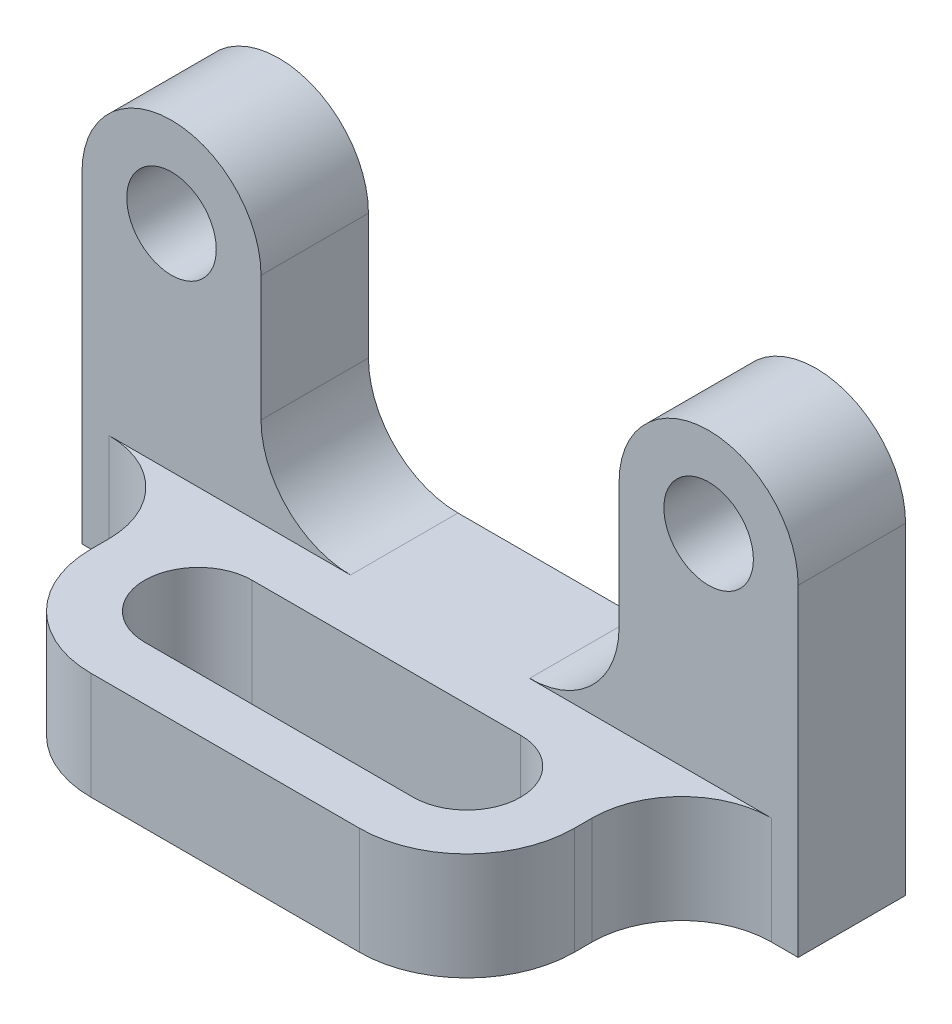
ISO-10303-21;
HEADER;
FILE_DESCRIPTION(('STEP AP214'),'2;1');
FILE_NAME('part.step','',(''),(''),'','','');
FILE_SCHEMA(('AUTOMOTIVE_DESIGN { 1 0 10303 214 1 1 1 1 }'));
ENDSEC;
DATA;
#1=APPLICATION_CONTEXT('core data for automotive mechanical design processes');
#2=APPLICATION_PROTOCOL_DEFINITION('international standard','automotive_design',2000,#1);
#3=PRODUCT_CONTEXT('',#1,'mechanical');
#4=PRODUCT('Part','Part','',(#3));
#5=PRODUCT_RELATED_PRODUCT_CATEGORY('part','',(#4));
#6=PRODUCT_DEFINITION_FORMATION('','',#4);
#7=PRODUCT_DEFINITION_CONTEXT('part definition',#1,'design');
#8=PRODUCT_DEFINITION('design','',#6,#7);
#9=PRODUCT_DEFINITION_SHAPE('','',#8);
#10=(LENGTH_UNIT() NAMED_UNIT(*) SI_UNIT(.MILLI.,.METRE.));
#11=(NAMED_UNIT(*) PLANE_ANGLE_UNIT() SI_UNIT($,.RADIAN.));
#12=(NAMED_UNIT(*) SI_UNIT($,.STERADIAN.) SOLID_ANGLE_UNIT());
#13=UNCERTAINTY_MEASURE_WITH_UNIT(LENGTH_MEASURE(1.E-05),#10,'distance_accuracy_value','');
#14=(GEOMETRIC_REPRESENTATION_CONTEXT(3) GLOBAL_UNCERTAINTY_ASSIGNED_CONTEXT((#13)) GLOBAL_UNIT_ASSIGNED_CONTEXT((#10,
#11,#12)) REPRESENTATION_CONTEXT('',''));
#15=CARTESIAN_POINT('',(0.,0.,0.));
#16=DIRECTION('',(0.,0.,1.));
#17=DIRECTION('',(1.,0.,0.));
#18=AXIS2_PLACEMENT_3D('',#15,#16,#17);
#19=CARTESIAN_POINT('',(0.,0.,6.));
#20=DIRECTION('',(0.,0.,1.));
#21=DIRECTION('',(1.,0.,0.));
#22=AXIS2_PLACEMENT_3D('',#19,#20,#21);
#23=PLANE('',#22);
#24=CARTESIAN_POINT('',(-15.,18.,6.));
#25=DIRECTION('',(0.,0.,1.));
#26=DIRECTION('',(1.,0.,0.));
#27=AXIS2_PLACEMENT_3D('',#24,#25,#26);
#28=CIRCLE('',#27,2.5);
#29=CARTESIAN_POINT('',(-12.5,18.,6.));
#30=VERTEX_POINT('',#29);
#31=EDGE_CURVE('E474',#30,#30,#28,.T.);
#32=ORIENTED_EDGE('',*,*,#31,.F.);
#33=EDGE_LOOP('',(#32));
#34=FACE_BOUND('',#33,.T.);
#35=DIRECTION('',(1.,0.,0.));
#36=VECTOR('',#35,1.);
#37=CARTESIAN_POINT('',(0.,0.,6.));
#38=LINE('',#37,#36);
#39=CARTESIAN_POINT('',(-20.,0.,6.));
#40=VERTEX_POINT('',#39);
#41=CARTESIAN_POINT('',(-18.5,0.,6.));
#42=VERTEX_POINT('',#41);
#43=EDGE_CURVE('E273',#40,#42,#38,.T.);
#44=ORIENTED_EDGE('',*,*,#43,.T.);
#45=DIRECTION('',(0.,-1.,0.));
#46=VECTOR('',#45,1.);
#47=CARTESIAN_POINT('',(-18.5,0.,6.));
#48=LINE('',#47,#46);
#49=CARTESIAN_POINT('',(-18.5,6.,6.));
#50=VERTEX_POINT('',#49);
#51=EDGE_CURVE('E359',#42,#50,#48,.F.);
#52=ORIENTED_EDGE('',*,*,#51,.T.);
#53=DIRECTION('',(-1.,0.,0.));
#54=VECTOR('',#53,1.);
#55=CARTESIAN_POINT('',(-13.5,6.,6.));
#56=LINE('',#55,#54);
#57=CARTESIAN_POINT('',(-5.,6.,6.));
#58=VERTEX_POINT('',#57);
#59=EDGE_CURVE('E243',#58,#50,#56,.T.);
#60=ORIENTED_EDGE('',*,*,#59,.F.);
#61=CARTESIAN_POINT('',(-5.,11.,6.));
#62=DIRECTION('',(0.,0.,1.));
#63=DIRECTION('',(1.,0.,0.));
#64=AXIS2_PLACEMENT_3D('',#61,#62,#63);
#65=CIRCLE('',#64,5.);
#66=CARTESIAN_POINT('',(-10.,11.,6.));
#67=VERTEX_POINT('',#66);
#68=EDGE_CURVE('E328',#58,#67,#65,.F.);
#69=ORIENTED_EDGE('',*,*,#68,.T.);
#70=DIRECTION('',(0.,-1.,0.));
#71=VECTOR('',#70,1.);
#72=CARTESIAN_POINT('',(-10.,0.,6.));
#73=LINE('',#72,#71);
#74=CARTESIAN_POINT('',(-10.,18.,6.));
#75=VERTEX_POINT('',#74);
#76=EDGE_CURVE('E264',#75,#67,#73,.T.);
#77=ORIENTED_EDGE('',*,*,#76,.F.);
#78=CARTESIAN_POINT('',(-15.,18.,6.));
#79=DIRECTION('',(0.,0.,1.));
#80=DIRECTION('',(1.,0.,0.));
#81=AXIS2_PLACEMENT_3D('',#78,#79,#80);
#82=CIRCLE('',#81,5.);
#83=CARTESIAN_POINT('',(-20.,18.,6.));
#84=VERTEX_POINT('',#83);
#85=EDGE_CURVE('E268',#75,#84,#82,.T.);
#86=ORIENTED_EDGE('',*,*,#85,.T.);
#87=DIRECTION('',(0.,1.,0.));
#88=VECTOR('',#87,1.);
#89=CARTESIAN_POINT('',(-20.,0.,6.));
#90=LINE('',#89,#88);
#91=EDGE_CURVE('E269',#40,#84,#90,.T.);
#92=ORIENTED_EDGE('',*,*,#91,.F.);
#93=EDGE_LOOP('',(#44,#52,#60,#69,#77,#86,#92));
#94=FACE_BOUND('',#93,.T.);
#95=ADVANCED_FACE('F44',(#34,#94),#23,.T.);
#96=CARTESIAN_POINT('',(20.,0.,6.));
#97=DIRECTION('',(-1.,0.,0.));
#98=DIRECTION('',(0.,0.,1.));
#99=AXIS2_PLACEMENT_3D('',#96,#97,#98);
#100=PLANE('',#99);
#101=DIRECTION('',(0.,1.,0.));
#102=VECTOR('',#101,1.);
#103=CARTESIAN_POINT('',(20.,0.,0.));
#104=LINE('',#103,#102);
#105=CARTESIAN_POINT('',(20.,0.,0.));
#106=VERTEX_POINT('',#105);
#107=CARTESIAN_POINT('',(20.,18.,0.));
#108=VERTEX_POINT('',#107);
#109=EDGE_CURVE('E254',#106,#108,#104,.T.);
#110=ORIENTED_EDGE('',*,*,#109,.T.);
#111=DIRECTION('',(0.,0.,-1.));
#112=VECTOR('',#111,1.);
#113=CARTESIAN_POINT('',(20.,18.,6.));
#114=LINE('',#113,#112);
#115=CARTESIAN_POINT('',(20.,18.,6.));
#116=VERTEX_POINT('',#115);
#117=EDGE_CURVE('E310',#116,#108,#114,.T.);
#118=ORIENTED_EDGE('',*,*,#117,.F.);
#119=DIRECTION('',(0.,1.,0.));
#120=VECTOR('',#119,1.);
#121=CARTESIAN_POINT('',(20.,0.,6.));
#122=LINE('',#121,#120);
#123=CARTESIAN_POINT('',(20.,0.,6.));
#124=VERTEX_POINT('',#123);
#125=EDGE_CURVE('E258',#124,#116,#122,.T.);
#126=ORIENTED_EDGE('',*,*,#125,.F.);
#127=DIRECTION('',(0.,0.,-1.));
#128=VECTOR('',#127,1.);
#129=CARTESIAN_POINT('',(20.,0.,6.));
#130=LINE('',#129,#128);
#131=EDGE_CURVE('E280',#124,#106,#130,.T.);
#132=ORIENTED_EDGE('',*,*,#131,.T.);
#133=EDGE_LOOP('',(#110,#118,#126,#132));
#134=FACE_BOUND('',#133,.T.);
#135=ADVANCED_FACE('F421',(#134),#100,.F.);
#136=CARTESIAN_POINT('',(15.,18.,6.));
#137=DIRECTION('',(0.,0.,-1.));
#138=DIRECTION('',(-1.,0.,0.));
#139=AXIS2_PLACEMENT_3D('',#136,#137,#138);
#140=CYLINDRICAL_SURFACE('',#139,5.);
#141=CARTESIAN_POINT('',(15.,18.,0.));
#142=DIRECTION('',(0.,0.,1.));
#143=DIRECTION('',(1.,0.,0.));
#144=AXIS2_PLACEMENT_3D('',#141,#142,#143);
#145=CIRCLE('',#144,5.);
#146=CARTESIAN_POINT('',(10.,18.,0.));
#147=VERTEX_POINT('',#146);
#148=EDGE_CURVE('E278',#108,#147,#145,.T.);
#149=ORIENTED_EDGE('',*,*,#148,.T.);
#150=DIRECTION('',(0.,0.,-1.));
#151=VECTOR('',#150,1.);
#152=CARTESIAN_POINT('',(10.,18.,6.));
#153=LINE('',#152,#151);
#154=CARTESIAN_POINT('',(10.,18.,6.));
#155=VERTEX_POINT('',#154);
#156=EDGE_CURVE('E308',#155,#147,#153,.T.);
#157=ORIENTED_EDGE('',*,*,#156,.F.);
#158=CARTESIAN_POINT('',(15.,18.,6.));
#159=DIRECTION('',(0.,0.,1.));
#160=DIRECTION('',(1.,0.,0.));
#161=AXIS2_PLACEMENT_3D('',#158,#159,#160);
#162=CIRCLE('',#161,5.);
#163=EDGE_CURVE('E259',#116,#155,#162,.T.);
#164=ORIENTED_EDGE('',*,*,#163,.F.);
#165=ORIENTED_EDGE('',*,*,#117,.T.);
#166=EDGE_LOOP('',(#149,#157,#164,#165));
#167=FACE_BOUND('',#166,.T.);
#168=ADVANCED_FACE('F416',(#167),#140,.T.);
#169=CARTESIAN_POINT('',(10.,0.,6.));
#170=DIRECTION('',(-1.,0.,0.));
#171=DIRECTION('',(0.,0.,1.));
#172=AXIS2_PLACEMENT_3D('',#169,#170,#171);
#173=PLANE('',#172);
#174=DIRECTION('',(0.,1.,0.));
#175=VECTOR('',#174,1.);
#176=CARTESIAN_POINT('',(10.,0.,0.));
#177=LINE('',#176,#175);
#178=CARTESIAN_POINT('',(10.,11.,0.));
#179=VERTEX_POINT('',#178);
#180=EDGE_CURVE('E283',#179,#147,#177,.T.);
#181=ORIENTED_EDGE('',*,*,#180,.F.);
#182=DIRECTION('',(0.,0.,-1.));
#183=VECTOR('',#182,1.);
#184=CARTESIAN_POINT('',(10.,11.,6.));
#185=LINE('',#184,#183);
#186=CARTESIAN_POINT('',(10.,11.,6.));
#187=VERTEX_POINT('',#186);
#188=EDGE_CURVE('E318',#179,#187,#185,.F.);
#189=ORIENTED_EDGE('',*,*,#188,.T.);
#190=DIRECTION('',(0.,1.,0.));
#191=VECTOR('',#190,1.);
#192=CARTESIAN_POINT('',(10.,0.,6.));
#193=LINE('',#192,#191);
#194=EDGE_CURVE('E263',#187,#155,#193,.T.);
#195=ORIENTED_EDGE('',*,*,#194,.T.);
#196=ORIENTED_EDGE('',*,*,#156,.T.);
#197=EDGE_LOOP('',(#181,#189,#195,#196));
#198=FACE_BOUND('',#197,.T.);
#199=ADVANCED_FACE('F411',(#198),#173,.T.);
#200=CARTESIAN_POINT('',(0.,6.,6.));
#201=DIRECTION('',(0.,1.,0.));
#202=DIRECTION('',(0.,0.,1.));
#203=AXIS2_PLACEMENT_3D('',#200,#201,#202);
#204=PLANE('',#203);
#205=CARTESIAN_POINT('',(-7.5,6.,12.));
#206=DIRECTION('',(0.,1.,0.));
#207=DIRECTION('',(0.,0.,1.));
#208=AXIS2_PLACEMENT_3D('',#205,#206,#207);
#209=CIRCLE('',#208,3.);
#210=CARTESIAN_POINT('',(-7.5,6.,9.));
#211=VERTEX_POINT('',#210);
#212=CARTESIAN_POINT('',(-7.5,6.,15.));
#213=VERTEX_POINT('',#212);
#214=EDGE_CURVE('E58',#211,#213,#209,.T.);
#215=ORIENTED_EDGE('',*,*,#214,.F.);
#216=DIRECTION('',(-1.,0.,0.));
#217=VECTOR('',#216,1.);
#218=CARTESIAN_POINT('',(-7.5,6.,9.));
#219=LINE('',#218,#217);
#220=CARTESIAN_POINT('',(7.5,6.,9.));
#221=VERTEX_POINT('',#220);
#222=EDGE_CURVE('E211',#221,#211,#219,.T.);
#223=ORIENTED_EDGE('',*,*,#222,.F.);
#224=CARTESIAN_POINT('',(7.5,6.,12.));
#225=DIRECTION('',(0.,1.,0.));
#226=DIRECTION('',(0.,0.,1.));
#227=AXIS2_PLACEMENT_3D('',#224,#225,#226);
#228=CIRCLE('',#227,3.);
#229=CARTESIAN_POINT('',(7.5,6.,15.));
#230=VERTEX_POINT('',#229);
#231=EDGE_CURVE('E212',#230,#221,#228,.T.);
#232=ORIENTED_EDGE('',*,*,#231,.F.);
#233=DIRECTION('',(1.,0.,0.));
#234=VECTOR('',#233,1.);
#235=CARTESIAN_POINT('',(-7.5,6.,15.));
#236=LINE('',#235,#234);
#237=EDGE_CURVE('E224',#213,#230,#236,.T.);
#238=ORIENTED_EDGE('',*,*,#237,.F.);
#239=EDGE_LOOP('',(#215,#223,#232,#238));
#240=FACE_BOUND('',#239,.T.);
#241=DIRECTION('',(0.,0.,-1.));
#242=VECTOR('',#241,1.);
#243=CARTESIAN_POINT('',(-13.5,6.,18.));
#244=LINE('',#243,#242);
#245=CARTESIAN_POINT('',(-13.5,6.,12.));
#246=VERTEX_POINT('',#245);
#247=CARTESIAN_POINT('',(-13.5,6.,11.));
#248=VERTEX_POINT('',#247);
#249=EDGE_CURVE('E238',#246,#248,#244,.T.);
#250=ORIENTED_EDGE('',*,*,#249,.F.);
#251=CARTESIAN_POINT('',(-7.5,6.,12.));
#252=DIRECTION('',(0.,1.,0.));
#253=DIRECTION('',(0.,0.,1.));
#254=AXIS2_PLACEMENT_3D('',#251,#252,#253);
#255=CIRCLE('',#254,6.);
#256=CARTESIAN_POINT('',(-7.5,6.,18.));
#257=VERTEX_POINT('',#256);
#258=EDGE_CURVE('E341',#246,#257,#255,.T.);
#259=ORIENTED_EDGE('',*,*,#258,.T.);
#260=DIRECTION('',(-1.,0.,0.));
#261=VECTOR('',#260,1.);
#262=CARTESIAN_POINT('',(-13.5,6.,18.));
#263=LINE('',#262,#261);
#264=CARTESIAN_POINT('',(7.5,6.,18.));
#265=VERTEX_POINT('',#264);
#266=EDGE_CURVE('E240',#265,#257,#263,.T.);
#267=ORIENTED_EDGE('',*,*,#266,.F.);
#268=CARTESIAN_POINT('',(7.5,6.,12.));
#269=DIRECTION('',(0.,1.,0.));
#270=DIRECTION('',(0.,0.,1.));
#271=AXIS2_PLACEMENT_3D('',#268,#269,#270);
#272=CIRCLE('',#271,6.);
#273=CARTESIAN_POINT('',(13.5,6.,12.));
#274=VERTEX_POINT('',#273);
#275=EDGE_CURVE('E342',#265,#274,#272,.T.);
#276=ORIENTED_EDGE('',*,*,#275,.T.);
#277=DIRECTION('',(0.,0.,-1.));
#278=VECTOR('',#277,1.);
#279=CARTESIAN_POINT('',(13.5,6.,18.));
#280=LINE('',#279,#278);
#281=CARTESIAN_POINT('',(13.5,6.,11.));
#282=VERTEX_POINT('',#281);
#283=EDGE_CURVE('E248',#274,#282,#280,.T.);
#284=ORIENTED_EDGE('',*,*,#283,.T.);
#285=CARTESIAN_POINT('',(18.5,6.,11.));
#286=DIRECTION('',(0.,1.,0.));
#287=DIRECTION('',(0.,0.,1.));
#288=AXIS2_PLACEMENT_3D('',#285,#286,#287);
#289=CIRCLE('',#288,5.);
#290=CARTESIAN_POINT('',(18.5,6.,6.));
#291=VERTEX_POINT('',#290);
#292=EDGE_CURVE('E356',#282,#291,#289,.F.);
#293=ORIENTED_EDGE('',*,*,#292,.T.);
#294=CARTESIAN_POINT('',(5.,6.,6.));
#295=VERTEX_POINT('',#294);
#296=EDGE_CURVE('E226',#291,#295,#56,.T.);
#297=ORIENTED_EDGE('',*,*,#296,.T.);
#298=DIRECTION('',(0.,0.,-1.));
#299=VECTOR('',#298,1.);
#300=CARTESIAN_POINT('',(5.,6.,0.));
#301=LINE('',#300,#299);
#302=CARTESIAN_POINT('',(5.,6.,0.));
#303=VERTEX_POINT('',#302);
#304=EDGE_CURVE('E312',#295,#303,#301,.T.);
#305=ORIENTED_EDGE('',*,*,#304,.T.);
#306=DIRECTION('',(1.,0.,0.));
#307=VECTOR('',#306,1.);
#308=CARTESIAN_POINT('',(0.,6.,0.));
#309=LINE('',#308,#307);
#310=CARTESIAN_POINT('',(-5.,6.,0.));
#311=VERTEX_POINT('',#310);
#312=EDGE_CURVE('E281',#311,#303,#309,.T.);
#313=ORIENTED_EDGE('',*,*,#312,.F.);
#314=DIRECTION('',(0.,0.,-1.));
#315=VECTOR('',#314,1.);
#316=CARTESIAN_POINT('',(-5.,6.,6.));
#317=LINE('',#316,#315);
#318=EDGE_CURVE('E315',#311,#58,#317,.F.);
#319=ORIENTED_EDGE('',*,*,#318,.T.);
#320=ORIENTED_EDGE('',*,*,#59,.T.);
#321=CARTESIAN_POINT('',(-18.5,6.,11.));
#322=DIRECTION('',(0.,1.,0.));
#323=DIRECTION('',(0.,0.,1.));
#324=AXIS2_PLACEMENT_3D('',#321,#322,#323);
#325=CIRCLE('',#324,5.);
#326=EDGE_CURVE('E11',#50,#248,#325,.F.);
#327=ORIENTED_EDGE('',*,*,#326,.T.);
#328=EDGE_LOOP('',(#250,#259,#267,#276,#284,#293,#297,#305,#313,#319,#320,#327));
#329=FACE_BOUND('',#328,.T.);
#330=ADVANCED_FACE('F374',(#240,#329),#204,.T.);
#331=CARTESIAN_POINT('',(-10.,0.,6.));
#332=DIRECTION('',(1.,0.,0.));
#333=DIRECTION('',(0.,0.,-1.));
#334=AXIS2_PLACEMENT_3D('',#331,#332,#333);
#335=PLANE('',#334);
#336=ORIENTED_EDGE('',*,*,#76,.T.);
#337=DIRECTION('',(0.,0.,-1.));
#338=VECTOR('',#337,1.);
#339=CARTESIAN_POINT('',(-10.,11.,0.));
#340=LINE('',#339,#338);
#341=CARTESIAN_POINT('',(-10.,11.,0.));
#342=VERTEX_POINT('',#341);
#343=EDGE_CURVE('E319',#67,#342,#340,.T.);
#344=ORIENTED_EDGE('',*,*,#343,.T.);
#345=DIRECTION('',(0.,-1.,0.));
#346=VECTOR('',#345,1.);
#347=CARTESIAN_POINT('',(-10.,0.,0.));
#348=LINE('',#347,#346);
#349=CARTESIAN_POINT('',(-10.,18.,0.));
#350=VERTEX_POINT('',#349);
#351=EDGE_CURVE('E287',#350,#342,#348,.T.);
#352=ORIENTED_EDGE('',*,*,#351,.F.);
#353=DIRECTION('',(0.,0.,-1.));
#354=VECTOR('',#353,1.);
#355=CARTESIAN_POINT('',(-10.,18.,6.));
#356=LINE('',#355,#354);
#357=EDGE_CURVE('E305',#75,#350,#356,.T.);
#358=ORIENTED_EDGE('',*,*,#357,.F.);
#359=EDGE_LOOP('',(#336,#344,#352,#358));
#360=FACE_BOUND('',#359,.T.);
#361=ADVANCED_FACE('F433',(#360),#335,.T.);
#362=CARTESIAN_POINT('',(-15.,18.,6.));
#363=DIRECTION('',(0.,0.,-1.));
#364=DIRECTION('',(-1.,0.,0.));
#365=AXIS2_PLACEMENT_3D('',#362,#363,#364);
#366=CYLINDRICAL_SURFACE('',#365,5.);
#367=CARTESIAN_POINT('',(-15.,18.,0.));
#368=DIRECTION('',(0.,0.,1.));
#369=DIRECTION('',(1.,0.,0.));
#370=AXIS2_PLACEMENT_3D('',#367,#368,#369);
#371=CIRCLE('',#370,5.);
#372=CARTESIAN_POINT('',(-20.,18.,0.));
#373=VERTEX_POINT('',#372);
#374=EDGE_CURVE('E292',#350,#373,#371,.T.);
#375=ORIENTED_EDGE('',*,*,#374,.T.);
#376=DIRECTION('',(0.,0.,-1.));
#377=VECTOR('',#376,1.);
#378=CARTESIAN_POINT('',(-20.,18.,6.));
#379=LINE('',#378,#377);
#380=EDGE_CURVE('E304',#84,#373,#379,.T.);
#381=ORIENTED_EDGE('',*,*,#380,.F.);
#382=ORIENTED_EDGE('',*,*,#85,.F.);
#383=ORIENTED_EDGE('',*,*,#357,.T.);
#384=EDGE_LOOP('',(#375,#381,#382,#383));
#385=FACE_BOUND('',#384,.T.);
#386=ADVANCED_FACE('F442',(#385),#366,.T.);
#387=CARTESIAN_POINT('',(-20.,0.,6.));
#388=DIRECTION('',(-1.,0.,0.));
#389=DIRECTION('',(0.,0.,1.));
#390=AXIS2_PLACEMENT_3D('',#387,#388,#389);
#391=PLANE('',#390);
#392=DIRECTION('',(0.,1.,0.));
#393=VECTOR('',#392,1.);
#394=CARTESIAN_POINT('',(-20.,0.,0.));
#395=LINE('',#394,#393);
#396=CARTESIAN_POINT('',(-20.,0.,0.));
#397=VERTEX_POINT('',#396);
#398=EDGE_CURVE('E294',#397,#373,#395,.T.);
#399=ORIENTED_EDGE('',*,*,#398,.F.);
#400=DIRECTION('',(0.,0.,-1.));
#401=VECTOR('',#400,1.);
#402=CARTESIAN_POINT('',(-20.,0.,6.));
#403=LINE('',#402,#401);
#404=EDGE_CURVE('E296',#40,#397,#403,.T.);
#405=ORIENTED_EDGE('',*,*,#404,.F.);
#406=ORIENTED_EDGE('',*,*,#91,.T.);
#407=ORIENTED_EDGE('',*,*,#380,.T.);
#408=EDGE_LOOP('',(#399,#405,#406,#407));
#409=FACE_BOUND('',#408,.T.);
#410=ADVANCED_FACE('F430',(#409),#391,.T.);
#411=CARTESIAN_POINT('',(0.,0.,6.));
#412=DIRECTION('',(0.,1.,0.));
#413=DIRECTION('',(0.,0.,1.));
#414=AXIS2_PLACEMENT_3D('',#411,#412,#413);
#415=PLANE('',#414);
#416=DIRECTION('',(-1.,0.,0.));
#417=VECTOR('',#416,1.);
#418=CARTESIAN_POINT('',(-7.5,0.,9.));
#419=LINE('',#418,#417);
#420=CARTESIAN_POINT('',(7.5,0.,9.));
#421=VERTEX_POINT('',#420);
#422=CARTESIAN_POINT('',(-7.5,0.,9.));
#423=VERTEX_POINT('',#422);
#424=EDGE_CURVE('E203',#421,#423,#419,.T.);
#425=ORIENTED_EDGE('',*,*,#424,.T.);
#426=CARTESIAN_POINT('',(-7.5,0.,12.));
#427=DIRECTION('',(0.,1.,0.));
#428=DIRECTION('',(0.,0.,1.));
#429=AXIS2_PLACEMENT_3D('',#426,#427,#428);
#430=CIRCLE('',#429,3.);
#431=CARTESIAN_POINT('',(-7.5,0.,15.));
#432=VERTEX_POINT('',#431);
#433=EDGE_CURVE('E191',#423,#432,#430,.T.);
#434=ORIENTED_EDGE('',*,*,#433,.T.);
#435=DIRECTION('',(1.,0.,0.));
#436=VECTOR('',#435,1.);
#437=CARTESIAN_POINT('',(-7.5,0.,15.));
#438=LINE('',#437,#436);
#439=CARTESIAN_POINT('',(7.5,0.,15.));
#440=VERTEX_POINT('',#439);
#441=EDGE_CURVE('E204',#432,#440,#438,.T.);
#442=ORIENTED_EDGE('',*,*,#441,.T.);
#443=CARTESIAN_POINT('',(7.5,0.,12.));
#444=DIRECTION('',(0.,1.,0.));
#445=DIRECTION('',(0.,0.,1.));
#446=AXIS2_PLACEMENT_3D('',#443,#444,#445);
#447=CIRCLE('',#446,3.);
#448=EDGE_CURVE('E67',#440,#421,#447,.T.);
#449=ORIENTED_EDGE('',*,*,#448,.T.);
#450=EDGE_LOOP('',(#425,#434,#442,#449));
#451=FACE_BOUND('',#450,.T.);
#452=DIRECTION('',(1.,0.,0.));
#453=VECTOR('',#452,1.);
#454=CARTESIAN_POINT('',(-13.5,0.,18.));
#455=LINE('',#454,#453);
#456=CARTESIAN_POINT('',(-7.5,0.,18.));
#457=VERTEX_POINT('',#456);
#458=CARTESIAN_POINT('',(7.5,0.,18.));
#459=VERTEX_POINT('',#458);
#460=EDGE_CURVE('E235',#457,#459,#455,.T.);
#461=ORIENTED_EDGE('',*,*,#460,.F.);
#462=CARTESIAN_POINT('',(-7.5,0.,12.));
#463=DIRECTION('',(0.,1.,0.));
#464=DIRECTION('',(0.,0.,1.));
#465=AXIS2_PLACEMENT_3D('',#462,#463,#464);
#466=CIRCLE('',#465,6.);
#467=CARTESIAN_POINT('',(-13.5,0.,12.));
#468=VERTEX_POINT('',#467);
#469=EDGE_CURVE('E339',#457,#468,#466,.F.);
#470=ORIENTED_EDGE('',*,*,#469,.T.);
#471=DIRECTION('',(0.,0.,-1.));
#472=VECTOR('',#471,1.);
#473=CARTESIAN_POINT('',(-13.5,0.,18.));
#474=LINE('',#473,#472);
#475=CARTESIAN_POINT('',(-13.5,0.,11.));
#476=VERTEX_POINT('',#475);
#477=EDGE_CURVE('E252',#468,#476,#474,.T.);
#478=ORIENTED_EDGE('',*,*,#477,.T.);
#479=CARTESIAN_POINT('',(-18.5,0.,11.));
#480=DIRECTION('',(0.,1.,0.));
#481=DIRECTION('',(0.,0.,1.));
#482=AXIS2_PLACEMENT_3D('',#479,#480,#481);
#483=CIRCLE('',#482,5.);
#484=EDGE_CURVE('E52',#476,#42,#483,.T.);
#485=ORIENTED_EDGE('',*,*,#484,.T.);
#486=ORIENTED_EDGE('',*,*,#43,.F.);
#487=ORIENTED_EDGE('',*,*,#404,.T.);
#488=DIRECTION('',(1.,0.,0.));
#489=VECTOR('',#488,1.);
#490=CARTESIAN_POINT('',(0.,0.,0.));
#491=LINE('',#490,#489);
#492=EDGE_CURVE('E257',#397,#106,#491,.T.);
#493=ORIENTED_EDGE('',*,*,#492,.T.);
#494=ORIENTED_EDGE('',*,*,#131,.F.);
#495=CARTESIAN_POINT('',(18.5,0.,6.));
#496=VERTEX_POINT('',#495);
#497=EDGE_CURVE('E272',#496,#124,#38,.T.);
#498=ORIENTED_EDGE('',*,*,#497,.F.);
#499=CARTESIAN_POINT('',(18.5,0.,11.));
#500=DIRECTION('',(0.,1.,0.));
#501=DIRECTION('',(0.,0.,1.));
#502=AXIS2_PLACEMENT_3D('',#499,#500,#501);
#503=CIRCLE('',#502,5.);
#504=CARTESIAN_POINT('',(13.5,0.,11.));
#505=VERTEX_POINT('',#504);
#506=EDGE_CURVE('E361',#496,#505,#503,.T.);
#507=ORIENTED_EDGE('',*,*,#506,.T.);
#508=DIRECTION('',(0.,0.,-1.));
#509=VECTOR('',#508,1.);
#510=CARTESIAN_POINT('',(13.5,0.,18.));
#511=LINE('',#510,#509);
#512=CARTESIAN_POINT('',(13.5,0.,12.));
#513=VERTEX_POINT('',#512);
#514=EDGE_CURVE('E250',#513,#505,#511,.T.);
#515=ORIENTED_EDGE('',*,*,#514,.F.);
#516=CARTESIAN_POINT('',(7.5,0.,12.));
#517=DIRECTION('',(0.,1.,0.));
#518=DIRECTION('',(0.,0.,1.));
#519=AXIS2_PLACEMENT_3D('',#516,#517,#518);
#520=CIRCLE('',#519,6.);
#521=EDGE_CURVE('E340',#513,#459,#520,.F.);
#522=ORIENTED_EDGE('',*,*,#521,.T.);
#523=EDGE_LOOP('',(#461,#470,#478,#485,#486,#487,#493,#494,#498,#507,#515,#522));
#524=FACE_BOUND('',#523,.T.);
#525=ADVANCED_FACE('F208',(#451,#524),#415,.F.);
#526=CARTESIAN_POINT('',(15.,18.,6.));
#527=DIRECTION('',(0.,0.,1.));
#528=DIRECTION('',(1.,0.,0.));
#529=AXIS2_PLACEMENT_3D('',#526,#527,#528);
#530=CIRCLE('',#529,2.5);
#531=CARTESIAN_POINT('',(17.5,18.,6.));
#532=VERTEX_POINT('',#531);
#533=EDGE_CURVE('E220',#532,#532,#530,.T.);
#534=ORIENTED_EDGE('',*,*,#533,.F.);
#535=EDGE_LOOP('',(#534));
#536=FACE_BOUND('',#535,.T.);
#537=ORIENTED_EDGE('',*,*,#296,.F.);
#538=DIRECTION('',(0.,1.,0.));
#539=VECTOR('',#538,1.);
#540=CARTESIAN_POINT('',(18.5,0.,6.));
#541=LINE('',#540,#539);
#542=EDGE_CURVE('E355',#291,#496,#541,.F.);
#543=ORIENTED_EDGE('',*,*,#542,.T.);
#544=ORIENTED_EDGE('',*,*,#497,.T.);
#545=ORIENTED_EDGE('',*,*,#125,.T.);
#546=ORIENTED_EDGE('',*,*,#163,.T.);
#547=ORIENTED_EDGE('',*,*,#194,.F.);
#548=CARTESIAN_POINT('',(5.,11.,6.));
#549=DIRECTION('',(0.,0.,1.));
#550=DIRECTION('',(1.,0.,0.));
#551=AXIS2_PLACEMENT_3D('',#548,#549,#550);
#552=CIRCLE('',#551,5.);
#553=EDGE_CURVE('E324',#187,#295,#552,.F.);
#554=ORIENTED_EDGE('',*,*,#553,.T.);
#555=EDGE_LOOP('',(#537,#543,#544,#545,#546,#547,#554));
#556=FACE_BOUND('',#555,.T.);
#557=ADVANCED_FACE('F401',(#536,#556),#23,.T.);
#558=CARTESIAN_POINT('',(0.,0.,0.));
#559=DIRECTION('',(0.,0.,1.));
#560=DIRECTION('',(1.,0.,0.));
#561=AXIS2_PLACEMENT_3D('',#558,#559,#560);
#562=PLANE('',#561);
#563=CARTESIAN_POINT('',(-15.,18.,0.));
#564=DIRECTION('',(0.,0.,1.));
#565=DIRECTION('',(1.,0.,0.));
#566=AXIS2_PLACEMENT_3D('',#563,#564,#565);
#567=CIRCLE('',#566,2.5);
#568=CARTESIAN_POINT('',(-12.5,18.,0.));
#569=VERTEX_POINT('',#568);
#570=EDGE_CURVE('E221',#569,#569,#567,.T.);
#571=ORIENTED_EDGE('',*,*,#570,.T.);
#572=EDGE_LOOP('',(#571));
#573=FACE_BOUND('',#572,.T.);
#574=CARTESIAN_POINT('',(15.,18.,0.));
#575=DIRECTION('',(0.,0.,1.));
#576=DIRECTION('',(1.,0.,0.));
#577=AXIS2_PLACEMENT_3D('',#574,#575,#576);
#578=CIRCLE('',#577,2.5);
#579=CARTESIAN_POINT('',(17.5,18.,0.));
#580=VERTEX_POINT('',#579);
#581=EDGE_CURVE('E471',#580,#580,#578,.T.);
#582=ORIENTED_EDGE('',*,*,#581,.T.);
#583=EDGE_LOOP('',(#582));
#584=FACE_BOUND('',#583,.T.);
#585=ORIENTED_EDGE('',*,*,#109,.F.);
#586=ORIENTED_EDGE('',*,*,#492,.F.);
#587=ORIENTED_EDGE('',*,*,#398,.T.);
#588=ORIENTED_EDGE('',*,*,#374,.F.);
#589=ORIENTED_EDGE('',*,*,#351,.T.);
#590=CARTESIAN_POINT('',(-5.,11.,0.));
#591=DIRECTION('',(0.,0.,1.));
#592=DIRECTION('',(1.,0.,0.));
#593=AXIS2_PLACEMENT_3D('',#590,#591,#592);
#594=CIRCLE('',#593,5.);
#595=EDGE_CURVE('E330',#342,#311,#594,.T.);
#596=ORIENTED_EDGE('',*,*,#595,.T.);
#597=ORIENTED_EDGE('',*,*,#312,.T.);
#598=CARTESIAN_POINT('',(5.,11.,0.));
#599=DIRECTION('',(0.,0.,1.));
#600=DIRECTION('',(1.,0.,0.));
#601=AXIS2_PLACEMENT_3D('',#598,#599,#600);
#602=CIRCLE('',#601,5.);
#603=EDGE_CURVE('E323',#303,#179,#602,.T.);
#604=ORIENTED_EDGE('',*,*,#603,.T.);
#605=ORIENTED_EDGE('',*,*,#180,.T.);
#606=ORIENTED_EDGE('',*,*,#148,.F.);
#607=EDGE_LOOP('',(#585,#586,#587,#588,#589,#596,#597,#604,#605,#606));
#608=FACE_BOUND('',#607,.T.);
#609=ADVANCED_FACE('F412',(#573,#584,#608),#562,.F.);
#610=CARTESIAN_POINT('',(5.,11.,6.));
#611=DIRECTION('',(0.,0.,1.));
#612=DIRECTION('',(1.,0.,0.));
#613=AXIS2_PLACEMENT_3D('',#610,#611,#612);
#614=CYLINDRICAL_SURFACE('',#613,5.);
#615=ORIENTED_EDGE('',*,*,#553,.F.);
#616=ORIENTED_EDGE('',*,*,#188,.F.);
#617=ORIENTED_EDGE('',*,*,#603,.F.);
#618=ORIENTED_EDGE('',*,*,#304,.F.);
#619=EDGE_LOOP('',(#615,#616,#617,#618));
#620=FACE_BOUND('',#619,.T.);
#621=ADVANCED_FACE('F409',(#620),#614,.F.);
#622=CARTESIAN_POINT('',(-5.,11.,6.));
#623=DIRECTION('',(0.,0.,1.));
#624=DIRECTION('',(1.,0.,0.));
#625=AXIS2_PLACEMENT_3D('',#622,#623,#624);
#626=CYLINDRICAL_SURFACE('',#625,5.);
#627=ORIENTED_EDGE('',*,*,#68,.F.);
#628=ORIENTED_EDGE('',*,*,#318,.F.);
#629=ORIENTED_EDGE('',*,*,#595,.F.);
#630=ORIENTED_EDGE('',*,*,#343,.F.);
#631=EDGE_LOOP('',(#627,#628,#629,#630));
#632=FACE_BOUND('',#631,.T.);
#633=ADVANCED_FACE('F438',(#632),#626,.F.);
#634=CARTESIAN_POINT('',(-13.5,0.,18.));
#635=DIRECTION('',(1.,0.,0.));
#636=DIRECTION('',(0.,0.,-1.));
#637=AXIS2_PLACEMENT_3D('',#634,#635,#636);
#638=PLANE('',#637);
#639=ORIENTED_EDGE('',*,*,#249,.T.);
#640=DIRECTION('',(0.,-1.,0.));
#641=VECTOR('',#640,1.);
#642=CARTESIAN_POINT('',(-13.5,0.,11.));
#643=LINE('',#642,#641);
#644=EDGE_CURVE('E354',#248,#476,#643,.T.);
#645=ORIENTED_EDGE('',*,*,#644,.T.);
#646=ORIENTED_EDGE('',*,*,#477,.F.);
#647=DIRECTION('',(0.,-1.,0.));
#648=VECTOR('',#647,1.);
#649=CARTESIAN_POINT('',(-13.5,0.,12.));
#650=LINE('',#649,#648);
#651=EDGE_CURVE('E343',#468,#246,#650,.F.);
#652=ORIENTED_EDGE('',*,*,#651,.T.);
#653=EDGE_LOOP('',(#639,#645,#646,#652));
#654=FACE_BOUND('',#653,.T.);
#655=ADVANCED_FACE('F378',(#654),#638,.F.);
#656=CARTESIAN_POINT('',(13.5,0.,18.));
#657=DIRECTION('',(-1.,0.,0.));
#658=DIRECTION('',(0.,-1.,0.));
#659=AXIS2_PLACEMENT_3D('',#656,#657,#658);
#660=PLANE('',#659);
#661=ORIENTED_EDGE('',*,*,#514,.T.);
#662=DIRECTION('',(0.,1.,0.));
#663=VECTOR('',#662,1.);
#664=CARTESIAN_POINT('',(13.5,0.,11.));
#665=LINE('',#664,#663);
#666=EDGE_CURVE('E349',#505,#282,#665,.T.);
#667=ORIENTED_EDGE('',*,*,#666,.T.);
#668=ORIENTED_EDGE('',*,*,#283,.F.);
#669=DIRECTION('',(0.,1.,0.));
#670=VECTOR('',#669,1.);
#671=CARTESIAN_POINT('',(13.5,0.,12.));
#672=LINE('',#671,#670);
#673=EDGE_CURVE('E350',#274,#513,#672,.F.);
#674=ORIENTED_EDGE('',*,*,#673,.T.);
#675=EDGE_LOOP('',(#661,#667,#668,#674));
#676=FACE_BOUND('',#675,.T.);
#677=ADVANCED_FACE('F393',(#676),#660,.F.);
#678=CARTESIAN_POINT('',(0.,0.,18.));
#679=DIRECTION('',(0.,0.,-1.));
#680=DIRECTION('',(-1.,0.,0.));
#681=AXIS2_PLACEMENT_3D('',#678,#679,#680);
#682=PLANE('',#681);
#683=ORIENTED_EDGE('',*,*,#266,.T.);
#684=DIRECTION('',(0.,-1.,0.));
#685=VECTOR('',#684,1.);
#686=CARTESIAN_POINT('',(-7.5,0.,18.));
#687=LINE('',#686,#685);
#688=EDGE_CURVE('E331',#257,#457,#687,.T.);
#689=ORIENTED_EDGE('',*,*,#688,.T.);
#690=ORIENTED_EDGE('',*,*,#460,.T.);
#691=DIRECTION('',(0.,1.,0.));
#692=VECTOR('',#691,1.);
#693=CARTESIAN_POINT('',(7.5,0.,18.));
#694=LINE('',#693,#692);
#695=EDGE_CURVE('E332',#459,#265,#694,.T.);
#696=ORIENTED_EDGE('',*,*,#695,.T.);
#697=EDGE_LOOP('',(#683,#689,#690,#696));
#698=FACE_BOUND('',#697,.T.);
#699=ADVANCED_FACE('F384',(#698),#682,.F.);
#700=CARTESIAN_POINT('',(-7.5,0.,12.));
#701=DIRECTION('',(0.,-1.,0.));
#702=DIRECTION('',(0.,0.,-1.));
#703=AXIS2_PLACEMENT_3D('',#700,#701,#702);
#704=CYLINDRICAL_SURFACE('',#703,6.);
#705=ORIENTED_EDGE('',*,*,#258,.F.);
#706=ORIENTED_EDGE('',*,*,#651,.F.);
#707=ORIENTED_EDGE('',*,*,#469,.F.);
#708=ORIENTED_EDGE('',*,*,#688,.F.);
#709=EDGE_LOOP('',(#705,#706,#707,#708));
#710=FACE_BOUND('',#709,.T.);
#711=ADVANCED_FACE('F381',(#710),#704,.T.);
#712=CARTESIAN_POINT('',(7.5,0.,12.));
#713=DIRECTION('',(0.,1.,0.));
#714=DIRECTION('',(-1.,0.,0.));
#715=AXIS2_PLACEMENT_3D('',#712,#713,#714);
#716=CYLINDRICAL_SURFACE('',#715,6.);
#717=ORIENTED_EDGE('',*,*,#521,.F.);
#718=ORIENTED_EDGE('',*,*,#673,.F.);
#719=ORIENTED_EDGE('',*,*,#275,.F.);
#720=ORIENTED_EDGE('',*,*,#695,.F.);
#721=EDGE_LOOP('',(#717,#718,#719,#720));
#722=FACE_BOUND('',#721,.T.);
#723=ADVANCED_FACE('F386',(#722),#716,.T.);
#724=CARTESIAN_POINT('',(18.5,0.,11.));
#725=DIRECTION('',(0.,1.,0.));
#726=DIRECTION('',(-1.,0.,0.));
#727=AXIS2_PLACEMENT_3D('',#724,#725,#726);
#728=CYLINDRICAL_SURFACE('',#727,5.);
#729=ORIENTED_EDGE('',*,*,#506,.F.);
#730=ORIENTED_EDGE('',*,*,#542,.F.);
#731=ORIENTED_EDGE('',*,*,#292,.F.);
#732=ORIENTED_EDGE('',*,*,#666,.F.);
#733=EDGE_LOOP('',(#729,#730,#731,#732));
#734=FACE_BOUND('',#733,.T.);
#735=ADVANCED_FACE('F397',(#734),#728,.F.);
#736=CARTESIAN_POINT('',(-18.5,0.,11.));
#737=DIRECTION('',(0.,-1.,0.));
#738=DIRECTION('',(0.,0.,-1.));
#739=AXIS2_PLACEMENT_3D('',#736,#737,#738);
#740=CYLINDRICAL_SURFACE('',#739,5.);
#741=ORIENTED_EDGE('',*,*,#326,.F.);
#742=ORIENTED_EDGE('',*,*,#51,.F.);
#743=ORIENTED_EDGE('',*,*,#484,.F.);
#744=ORIENTED_EDGE('',*,*,#644,.F.);
#745=EDGE_LOOP('',(#741,#742,#743,#744));
#746=FACE_BOUND('',#745,.T.);
#747=ADVANCED_FACE('F50',(#746),#740,.F.);
#748=CARTESIAN_POINT('',(-7.5,0.,12.));
#749=DIRECTION('',(0.,1.,0.));
#750=DIRECTION('',(0.,0.,1.));
#751=AXIS2_PLACEMENT_3D('',#748,#749,#750);
#752=CYLINDRICAL_SURFACE('',#751,3.);
#753=ORIENTED_EDGE('',*,*,#214,.T.);
#754=DIRECTION('',(0.,1.,0.));
#755=VECTOR('',#754,1.);
#756=CARTESIAN_POINT('',(-7.5,0.,15.));
#757=LINE('',#756,#755);
#758=EDGE_CURVE('E193',#432,#213,#757,.T.);
#759=ORIENTED_EDGE('',*,*,#758,.F.);
#760=ORIENTED_EDGE('',*,*,#433,.F.);
#761=DIRECTION('',(0.,1.,0.));
#762=VECTOR('',#761,1.);
#763=CARTESIAN_POINT('',(-7.5,0.,9.));
#764=LINE('',#763,#762);
#765=EDGE_CURVE('E228',#423,#211,#764,.T.);
#766=ORIENTED_EDGE('',*,*,#765,.T.);
#767=EDGE_LOOP('',(#753,#759,#760,#766));
#768=FACE_BOUND('',#767,.T.);
#769=ADVANCED_FACE('F192',(#768),#752,.F.);
#770=CARTESIAN_POINT('',(-7.5,0.,9.));
#771=DIRECTION('',(0.,0.,-1.));
#772=DIRECTION('',(-1.,0.,0.));
#773=AXIS2_PLACEMENT_3D('',#770,#771,#772);
#774=PLANE('',#773);
#775=ORIENTED_EDGE('',*,*,#222,.T.);
#776=ORIENTED_EDGE('',*,*,#765,.F.);
#777=ORIENTED_EDGE('',*,*,#424,.F.);
#778=DIRECTION('',(0.,1.,0.));
#779=VECTOR('',#778,1.);
#780=CARTESIAN_POINT('',(7.5,0.,9.));
#781=LINE('',#780,#779);
#782=EDGE_CURVE('E233',#421,#221,#781,.T.);
#783=ORIENTED_EDGE('',*,*,#782,.T.);
#784=EDGE_LOOP('',(#775,#776,#777,#783));
#785=FACE_BOUND('',#784,.T.);
#786=ADVANCED_FACE('F494',(#785),#774,.F.);
#787=CARTESIAN_POINT('',(7.5,0.,12.));
#788=DIRECTION('',(0.,1.,0.));
#789=DIRECTION('',(0.,0.,1.));
#790=AXIS2_PLACEMENT_3D('',#787,#788,#789);
#791=CYLINDRICAL_SURFACE('',#790,3.);
#792=ORIENTED_EDGE('',*,*,#231,.T.);
#793=ORIENTED_EDGE('',*,*,#782,.F.);
#794=ORIENTED_EDGE('',*,*,#448,.F.);
#795=DIRECTION('',(0.,1.,0.));
#796=VECTOR('',#795,1.);
#797=CARTESIAN_POINT('',(7.5,0.,15.));
#798=LINE('',#797,#796);
#799=EDGE_CURVE('E199',#440,#230,#798,.T.);
#800=ORIENTED_EDGE('',*,*,#799,.T.);
#801=EDGE_LOOP('',(#792,#793,#794,#800));
#802=FACE_BOUND('',#801,.T.);
#803=ADVANCED_FACE('F499',(#802),#791,.F.);
#804=CARTESIAN_POINT('',(-7.5,0.,15.));
#805=DIRECTION('',(0.,0.,1.));
#806=DIRECTION('',(1.,0.,0.));
#807=AXIS2_PLACEMENT_3D('',#804,#805,#806);
#808=PLANE('',#807);
#809=ORIENTED_EDGE('',*,*,#237,.T.);
#810=ORIENTED_EDGE('',*,*,#799,.F.);
#811=ORIENTED_EDGE('',*,*,#441,.F.);
#812=ORIENTED_EDGE('',*,*,#758,.T.);
#813=EDGE_LOOP('',(#809,#810,#811,#812));
#814=FACE_BOUND('',#813,.T.);
#815=ADVANCED_FACE('F202',(#814),#808,.F.);
#816=CARTESIAN_POINT('',(15.,18.,0.));
#817=DIRECTION('',(0.,0.,1.));
#818=DIRECTION('',(1.,0.,0.));
#819=AXIS2_PLACEMENT_3D('',#816,#817,#818);
#820=CYLINDRICAL_SURFACE('',#819,2.5);
#821=ORIENTED_EDGE('',*,*,#581,.F.);
#822=EDGE_LOOP('',(#821));
#823=FACE_BOUND('',#822,.T.);
#824=ORIENTED_EDGE('',*,*,#533,.T.);
#825=EDGE_LOOP('',(#824));
#826=FACE_BOUND('',#825,.T.);
#827=ADVANCED_FACE('F490',(#823,#826),#820,.F.);
#828=CARTESIAN_POINT('',(-15.,18.,0.));
#829=DIRECTION('',(0.,0.,1.));
#830=DIRECTION('',(1.,0.,0.));
#831=AXIS2_PLACEMENT_3D('',#828,#829,#830);
#832=CYLINDRICAL_SURFACE('',#831,2.5);
#833=ORIENTED_EDGE('',*,*,#570,.F.);
#834=EDGE_LOOP('',(#833));
#835=FACE_BOUND('',#834,.T.);
#836=ORIENTED_EDGE('',*,*,#31,.T.);
#837=EDGE_LOOP('',(#836));
#838=FACE_BOUND('',#837,.T.);
#839=ADVANCED_FACE('F482',(#835,#838),#832,.F.);
#840=CLOSED_SHELL('',(#95,#135,#168,#199,#330,#361,#386,#410,#525,#557,#609,#621,#633,#655,#677,
#699,#711,#723,#735,#747,#769,#786,#803,#815,#827,#839));
#841=MANIFOLD_SOLID_BREP('B2',#840);
#842=ADVANCED_BREP_SHAPE_REPRESENTATION('',(#18,#841),#14);
#843=SHAPE_DEFINITION_REPRESENTATION(#9,#842);
ENDSEC;
END-ISO-10303-21;
